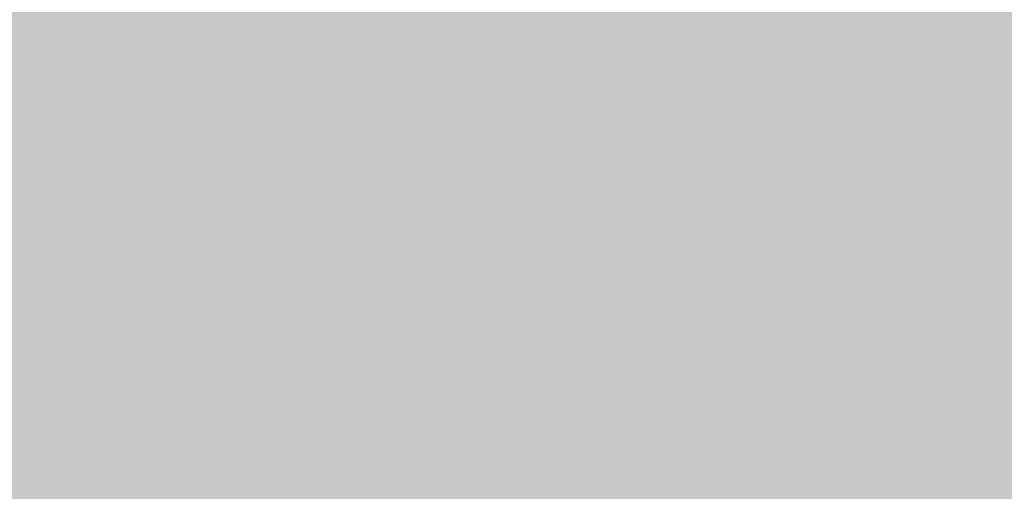
# Model space of a CAD drawing. Units: millimetres. Extents: x 0 to 2267, y 0 to 1823.
# Tile 201 of 256: x 1838.83 to 1841.442, y 1128.399 to 1129.649. Entities that reach past the tile are written whole.
import ezdxf

# ---------------------------------------------------------------- set-up
doc = ezdxf.new("R2010")
doc.units = ezdxf.units.MM
doc.header["$MEASUREMENT"] = 0
doc.layers.add('M-HATC', color=252, linetype='Continuous', lineweight=18)

msp = doc.modelspace()

# ---------------------------------------------------------------- hatches: boundary and pattern name
at = {"layer": 'M-HATC'}
h = msp.add_hatch(color=256, dxfattribs=at)
h.dxf.hatch_style = 1
h.paths.add_polyline_path([(2055.771, 1603.062), (1381.0868, 1603.062), (1381.0868, 1598.062), (2055.771, 1598.062)])
h.paths.add_polyline_path([(2055.771, 1598.062), (1381.0868, 1598.062), (1381.0868, 1593.062), (2055.771, 1593.062)])
h.paths.add_polyline_path([(2051.3074, 1536.7609), (1385.5504, 1536.7609), (1385.5504, 1526.7609), (1387.5504, 1526.7609), (1388.5366, 1525.0528), (1385.3319, 1521.2335), (1385.3319, 1521.2226), (2050.2542, 1522.7491), (2048.3212, 1525.0528), (2049.3074, 1526.7609), (2051.3074, 1526.7609)])
edge = h.paths.add_edge_path()
edge.add_arc((1847.5345, 1379.1492), 135, 222.603061, 222.890851, ccw=False)
edge.add_line((1748.1663, 1287.7656), (1683.0921, 1287.7656))
edge.add_arc((1583.7239, 1379.1492), 135, 317.109149, 317.396939, ccw=False)
edge.add_arc((1678.9686, 1290.6707), 5, 222.8909, 317.1091, ccw=False)
edge.add_arc((1774.2133, 1379.1492), 135, 222.603061, 222.890851, ccw=False)
edge.add_line((1674.8451, 1287.7656), (1609.7709, 1287.7656))
edge.add_arc((1510.4027, 1379.1492), 135, 317.109149, 317.396939, ccw=False)
edge.add_arc((1605.6474, 1290.6707), 5, 222.8909, 317.1091, ccw=False)
edge.add_arc((1700.8921, 1379.1492), 135, 222.603061, 222.890851, ccw=False)
edge.add_line((1601.5239, 1287.7656), (1536.4497, 1287.7656))
edge.add_arc((1437.0815, 1379.1492), 135, 317.109149, 317.396939, ccw=False)
edge.add_arc((1532.3262, 1290.6707), 5, 222.8909, 317.1091, ccw=False)
edge.add_arc((1627.5709, 1379.1492), 135, 222.603061, 222.890851, ccw=False)
edge.add_line((1528.2027, 1287.7656), (1505.9289, 1287.7656))
edge.add_spline(control_points=[(1505.9289, 1287.7656), (1504.2622, 1287.7656), (1504.2622, 1282.7656), (1505.9289, 1282.7656)], knot_values=[0, 0, 0, 0, 5, 5, 5, 5], degree=3, periodic=0)
edge.add_line((1505.9289, 1282.7656), (1930.9289, 1282.7656))
edge.add_spline(control_points=[(1930.9289, 1282.7656), (1932.5956, 1282.7656), (1932.5956, 1287.7656), (1930.9289, 1287.7656)], knot_values=[0, 0, 0, 0, 5, 5, 5, 5], degree=3, periodic=0)
edge.add_line((1930.9289, 1287.7656), (1903.0557, 1287.7656))
edge.add_arc((1803.6875, 1379.1492), 135, 317.109149, 317.396939, ccw=False)
edge.add_arc((1898.9322, 1290.6707), 5, 222.8909, 317.1091, ccw=False)
edge.add_arc((1994.1769, 1379.1492), 135, 222.603061, 222.890851, ccw=False)
edge.add_line((1894.8087, 1287.7656), (1829.7345, 1287.7656))
edge.add_arc((1730.3663, 1379.1492), 135, 317.109149, 317.396939, ccw=False)
edge.add_arc((1825.611, 1290.6707), 5, 222.8909, 317.1091, ccw=False)
edge.add_arc((1920.8557, 1379.1492), 135, 222.603061, 222.890851, ccw=False)
edge.add_line((1821.4875, 1287.7656), (1756.4133, 1287.7656))
edge.add_arc((1657.0451, 1379.1492), 135, 317.109149, 317.396939, ccw=False)
edge.add_arc((1752.2898, 1290.6707), 5, 222.8909, 317.1091, ccw=False)
edge = h.paths.add_edge_path()
edge.add_spline(control_points=[(1843.4289, 1227.2475), (1845.0956, 1227.2475), (1845.0956, 1232.2475), (1843.4289, 1232.2475)], knot_values=[0, 0, 0, 0, 5, 5, 5, 5], degree=3, periodic=0)
edge.add_line((1843.4289, 1232.2475), (1593.4289, 1232.2475))
edge.add_spline(control_points=[(1593.4289, 1232.2475), (1591.7622, 1232.2475), (1591.7622, 1227.2475), (1593.4289, 1227.2475)], knot_values=[0, 0, 0, 0, 5, 5, 5, 5], degree=3, periodic=0)
edge.add_line((1593.4289, 1227.2475), (1843.4289, 1227.2475))
h.paths.add_polyline_path([(1905.9289, 1127.4171), (1530.9289, 1127.4171, 0.414214), (1520.9289, 1117.4171), (1530.9289, 1117.4171), (1915.9289, 1117.4171, 0.414214)])
edge = h.paths.add_edge_path()
edge.add_arc((1397.0858, 1498.4078), 12.7299, 90.78215, 190.87871, ccw=False)
edge.add_line((1396.912, 1511.1365), (1428.0097, 1511.3488))
edge.add_line((1428.0097, 1511.3488), (1433.0097, 1511.3488))
edge.add_line((1433.0097, 1511.3488), (1434.439, 1511.3488))
edge.add_arc((1419.474, 1498.0804), 20, 41.561, 74.08211)
edge.add_line((1424.9592, 1517.3135), (1399.9351, 1517.2561))
edge.add_spline(control_points=[(1399.9307, 1517.2561), (1399.884, 1517.2131), (1399.8328, 1517.1689), (1399.7774, 1517.1236)], knot_values=[11.567499, 11.567499, 11.567499, 11.567499, 11.814249, 11.814249, 11.814249, 11.814249], degree=3, periodic=0)
edge.add_spline(control_points=[(1399.6328, 1517.0099), (1399.5831, 1516.9721), (1399.5307, 1516.9338), (1399.4759, 1516.8947)], knot_values=[11.167718, 11.167718, 11.167718, 11.167718, 11.365188, 11.365188, 11.365188, 11.365188], degree=3, periodic=0)
edge.add_spline(control_points=[(1399.3398, 1516.8001), (1399.1514, 1516.6719), (1398.9384, 1516.5377), (1398.704, 1516.3994)], knot_values=[10.376405, 10.376405, 10.376405, 10.376405, 11.00994, 11.00994, 11.00994, 11.00994], degree=3, periodic=0)
edge.add_spline(control_points=[(1398.6572, 1516.3719), (1398.5789, 1516.326), (1398.4983, 1516.2797), (1398.4155, 1516.2331)], knot_values=[10.125175, 10.125175, 10.125175, 10.125175, 10.334406, 10.334406, 10.334406, 10.334406], degree=3, periodic=0)
edge.add_spline(control_points=[(1398.2642, 1516.1487), (1398.196, 1516.1111), (1398.1263, 1516.0732), (1398.0555, 1516.0351)], knot_values=[9.832246, 9.832246, 9.832246, 9.832246, 9.999658, 9.999658, 9.999658, 9.999658], degree=3, periodic=0)
edge.add_spline(control_points=[(1397.9987, 1516.0048), (1397.7312, 1515.8621), (1397.446, 1515.7171), (1397.1466, 1515.5714)], knot_values=[9.161808, 9.161808, 9.161808, 9.161808, 9.787769, 9.787769, 9.787769, 9.787769], degree=3, periodic=0)
edge.add_spline(control_points=[(1397.1466, 1515.5714), (1396.8418, 1515.423), (1396.5222, 1515.274), (1396.1914, 1515.1262)], knot_values=[8.524455, 8.524455, 8.524455, 8.524455, 9.161808, 9.161808, 9.161808, 9.161808], degree=3, periodic=0)
edge.add_spline(control_points=[(1396.0777, 1515.0756), (1395.9854, 1515.0348), (1395.8922, 1514.994), (1395.7983, 1514.9534)], knot_values=[8.275193, 8.275193, 8.275193, 8.275193, 8.451726, 8.451726, 8.451726, 8.451726], degree=3, periodic=0)
edge.add_spline(control_points=[(1395.6018, 1514.8691), (1395.4997, 1514.8257), (1395.3968, 1514.7824), (1395.2932, 1514.7394)], knot_values=[7.962917, 7.962917, 7.962917, 7.962917, 8.152764, 8.152764, 8.152764, 8.152764], degree=3, periodic=0)
edge.add_spline(control_points=[(1395.2116, 1514.7057), (1394.8278, 1514.5475), (1394.4345, 1514.3929), (1394.0364, 1514.2442)], knot_values=[7.21254, 7.21254, 7.21254, 7.21254, 7.913148, 7.913148, 7.913148, 7.913148], degree=3, periodic=0)
edge.add_spline(control_points=[(1394.0364, 1514.2442), (1393.7076, 1514.1214), (1393.3754, 1514.0027), (1393.0427, 1513.8895)], knot_values=[6.633733, 6.633733, 6.633733, 6.633733, 7.21254, 7.21254, 7.21254, 7.21254], degree=3, periodic=0)
edge.add_spline(control_points=[(1392.8214, 1513.815), (1392.7198, 1513.7812), (1392.6181, 1513.7479), (1392.5166, 1513.7152)], knot_values=[6.328796, 6.328796, 6.328796, 6.328796, 6.505493, 6.505493, 6.505493, 6.505493], degree=3, periodic=0)
edge.add_spline(control_points=[(1392.5166, 1513.7152), (1392.3187, 1513.6515), (1392.1212, 1513.59), (1391.9244, 1513.531)], knot_values=[5.984605, 5.984605, 5.984605, 5.984605, 6.328796, 6.328796, 6.328796, 6.328796], degree=3, periodic=0)
edge.add_spline(control_points=[(1391.7915, 1513.4915), (1391.3122, 1513.3501), (1390.8384, 1513.2239), (1390.3784, 1513.1171)], knot_values=[5.066697, 5.066697, 5.066697, 5.066697, 5.907055, 5.907055, 5.907055, 5.907055], degree=3, periodic=0)
edge.add_spline(control_points=[(1390.3784, 1513.1171), (1390.1797, 1513.071), (1389.9836, 1513.0284), (1389.7907, 1512.9899)], knot_values=[4.70367, 4.70367, 4.70367, 4.70367, 5.066695, 5.066695, 5.066695, 5.066695], degree=3, periodic=0)
edge.add_spline(control_points=[(1389.422, 1512.9204), (1389.2459, 1512.8892), (1389.0729, 1512.8617), (1388.9036, 1512.8381)], knot_values=[4.130571, 4.130571, 4.130571, 4.130571, 4.469816, 4.469816, 4.469816, 4.469816], degree=3, periodic=0)
edge.add_spline(control_points=[(1388.9036, 1512.8381), (1388.591, 1512.7946), (1388.2911, 1512.7644), (1388.0071, 1512.7494)], knot_values=[3.504031, 3.504031, 3.504031, 3.504031, 4.130571, 4.130571, 4.130571, 4.130571], degree=3, periodic=0)
edge.add_spline(control_points=[(1387.9356, 1512.7459), (1387.8538, 1512.7423), (1387.7733, 1512.74), (1387.6944, 1512.739)], knot_values=[3.268866, 3.268866, 3.268866, 3.268866, 3.451164, 3.451164, 3.451164, 3.451164], degree=3, periodic=0)
edge.add_spline(control_points=[(1387.3351, 1512.7443), (1387.2076, 1512.7499), (1387.0847, 1512.7597), (1386.967, 1512.7739)], knot_values=[2.670686, 2.670686, 2.670686, 2.670686, 2.984, 2.984, 2.984, 2.984], degree=3, periodic=0)
edge.add_spline(control_points=[(1386.8327, 1512.7922), (1386.8209, 1512.7941), (1386.8092, 1512.7959), (1386.7975, 1512.7979)], knot_values=[2.516981, 2.516981, 2.516981, 2.516981, 2.549528, 2.549528, 2.549528, 2.549528], degree=3, periodic=0)
edge.add_spline(control_points=[(1386.4526, 1512.8735), (1386.4257, 1512.881), (1386.3993, 1512.889), (1386.3733, 1512.8972)], knot_values=[2.095869, 2.095869, 2.095869, 2.095869, 2.17941, 2.17941, 2.17941, 2.17941], degree=3, periodic=0)
edge.add_spline(control_points=[(1386.0691, 1513.0189), (1386.0634, 1513.0217), (1386.0577, 1513.0246), (1386.052, 1513.0275)], knot_values=[1.72453, 1.72453, 1.72453, 1.72453, 1.745933, 1.745933, 1.745933, 1.745933], degree=3, periodic=0)
edge.add_arc((1399.474, 1498.0804), 20, 131.82432, 180)
edge.add_arc((1630.3336, 1505.5484), 250.9708, 181.705176, 236.427975)
edge.add_arc((1605.3399, 1483.3044), 218.7822, 238.660829, 243.34961)
edge.add_arc((1647.0911, 1510.3592), 262.8986, 183.129836, 237.853442, ccw=False)
h.paths.add_polyline_path([(1406.5369, 1391.9644, 0.149382), (1491.5506, 1296.4418, -0.129517)], flags=17)
edge = h.paths.add_edge_path()
edge.add_arc((2037.3838, 1498.0804), 20, 0, 48.26587)
edge.add_spline(control_points=[(2050.6973, 1513.0052), (2050.6512, 1512.9847), (2050.6034, 1512.9655), (2050.5539, 1512.9477)], knot_values=[1.835652, 1.835652, 1.835652, 1.835652, 2.000781, 2.000781, 2.000781, 2.000781], degree=3, periodic=0)
edge.add_spline(control_points=[(2050.4616, 1512.9166), (2050.479, 1512.9221), (2050.4963, 1512.9277), (2050.5133, 1512.9335)], knot_values=[2.045477, 2.045477, 2.045477, 2.045477, 2.101389, 2.101389, 2.101389, 2.101389], degree=3, periodic=0)
edge.add_spline(control_points=[(2050.129, 1512.8342), (2050.1984, 1512.8473), (2050.2657, 1512.8623), (2050.3308, 1512.8792)], knot_values=[2.237629, 2.237629, 2.237629, 2.237629, 2.435841, 2.435841, 2.435841, 2.435841], degree=3, periodic=0)
edge.add_spline(control_points=[(2050.0946, 1512.8278), (2050.1061, 1512.8299), (2050.1176, 1512.832), (2050.129, 1512.8342)], knot_values=[2.435841, 2.435841, 2.435841, 2.435841, 2.468321, 2.468321, 2.468321, 2.468321], degree=3, periodic=0)
edge.add_spline(control_points=[(2049.7843, 1512.7851), (2049.8552, 1512.7922), (2049.9243, 1512.8008), (2049.9917, 1512.8109)], knot_values=[2.563852, 2.563852, 2.563852, 2.563852, 2.748541, 2.748541, 2.748541, 2.748541], degree=3, periodic=0)
edge.add_spline(control_points=[(2049.4052, 1512.7617), (2049.5364, 1512.7653), (2049.6629, 1512.773), (2049.7843, 1512.7851)], knot_values=[2.748541, 2.748541, 2.748541, 2.748541, 3.064882, 3.064882, 3.064882, 3.064882], degree=3, periodic=0)
edge.add_spline(control_points=[(2049.1698, 1512.7597), (2049.2336, 1512.7591), (2049.2965, 1512.7594), (2049.3584, 1512.7606)], knot_values=[3.102309, 3.102309, 3.102309, 3.102309, 3.2503, 3.2503, 3.2503, 3.2503], degree=3, periodic=0)
edge.add_spline(control_points=[(2048.8573, 1512.7691), (2048.9638, 1512.7638), (2049.068, 1512.7606), (2049.1698, 1512.7597)], knot_values=[3.2503, 3.2503, 3.2503, 3.2503, 3.486069, 3.486069, 3.486069, 3.486069], degree=3, periodic=0)
edge.add_spline(control_points=[(2048.6924, 1512.7789), (2048.3729, 1512.8009), (2048.0345, 1512.8411), (2047.6817, 1512.897)], knot_values=[3.606429, 3.606429, 3.606429, 3.606429, 4.2989, 4.2989, 4.2989, 4.2989], degree=3, periodic=0)
edge.add_spline(control_points=[(2047.6817, 1512.897), (2047.5458, 1512.9185), (2047.4077, 1512.9424), (2047.2678, 1512.9685)], knot_values=[4.2989, 4.2989, 4.2989, 4.2989, 4.565769, 4.565769, 4.565769, 4.565769], degree=3, periodic=0)
edge.add_spline(control_points=[(2047.2678, 1512.9685), (2047.1449, 1512.9914), (2047.0207, 1513.016), (2046.8951, 1513.0422)], knot_values=[4.565769, 4.565769, 4.565769, 4.565769, 4.799971, 4.799971, 4.799971, 4.799971], degree=3, periodic=0)
edge.add_spline(control_points=[(2046.8951, 1513.0422), (2046.5286, 1513.1188), (2046.1513, 1513.209), (2045.7676, 1513.3107)], knot_values=[4.799971, 4.799971, 4.799971, 4.799971, 5.483718, 5.483718, 5.483718, 5.483718], degree=3, periodic=0)
edge.add_spline(control_points=[(2045.7676, 1513.3107), (2045.3724, 1513.4154), (2044.9704, 1513.5322), (2044.5662, 1513.6588)], knot_values=[5.483718, 5.483718, 5.483718, 5.483718, 6.187866, 6.187866, 6.187866, 6.187866], degree=3, periodic=0)
edge.add_spline(control_points=[(2044.5662, 1513.6588), (2044.4149, 1513.7061), (2044.2633, 1513.7549), (2044.1116, 1513.8048)], knot_values=[6.187866, 6.187866, 6.187866, 6.187866, 6.451551, 6.451551, 6.451551, 6.451551], degree=3, periodic=0)
edge.add_spline(control_points=[(2044.1116, 1513.8048), (2043.9967, 1513.8427), (2043.8817, 1513.8813), (2043.7668, 1513.9205)], knot_values=[6.451551, 6.451551, 6.451551, 6.451551, 6.651434, 6.651434, 6.651434, 6.651434], degree=3, periodic=0)
edge.add_spline(control_points=[(2043.7668, 1513.9205), (2043.3716, 1514.0554), (2042.9774, 1514.1979), (2042.5886, 1514.3458)], knot_values=[6.651434, 6.651434, 6.651434, 6.651434, 7.338879, 7.338879, 7.338879, 7.338879], degree=3, periodic=0)
edge.add_spline(control_points=[(2042.5886, 1514.3458), (2042.1643, 1514.5071), (2041.7465, 1514.6749), (2041.3409, 1514.846)], knot_values=[7.338879, 7.338879, 7.338879, 7.338879, 8.089209, 8.089209, 8.089209, 8.089209], degree=3, periodic=0)
edge.add_spline(control_points=[(2041.3409, 1514.846), (2041.1028, 1514.9465), (2040.869, 1515.0481), (2040.6405, 1515.1502)], knot_values=[8.089209, 8.089209, 8.089209, 8.089209, 8.529587, 8.529587, 8.529587, 8.529587], degree=3, periodic=0)
edge.add_spline(control_points=[(2040.51, 1515.2089), (2040.0824, 1515.4022), (2039.6747, 1515.5971), (2039.295, 1515.7894)], knot_values=[8.613818, 8.613818, 8.613818, 8.613818, 9.44571, 9.44571, 9.44571, 9.44571], degree=3, periodic=0)
edge.add_spline(control_points=[(2039.295, 1515.7894), (2039.0618, 1515.9075), (2038.8391, 1516.0246), (2038.6288, 1516.1398)], knot_values=[9.44571, 9.44571, 9.44571, 9.44571, 9.956404, 9.956404, 9.956404, 9.956404], degree=3, periodic=0)
edge.add_spline(control_points=[(2038.6288, 1516.1398), (2038.5187, 1516.2001), (2038.4121, 1516.2598), (2038.309, 1516.3189)], knot_values=[9.956404, 9.956404, 9.956404, 9.956404, 10.223542, 10.223542, 10.223542, 10.223542], degree=3, periodic=0)
edge.add_spline(control_points=[(2038.309, 1516.3189), (2038.2138, 1516.3735), (2038.1216, 1516.4276), (2038.0328, 1516.481)], knot_values=[10.223542, 10.223542, 10.223542, 10.223542, 10.47051, 10.47051, 10.47051, 10.47051], degree=3, periodic=0)
edge.add_spline(control_points=[(2038.0328, 1516.481), (2037.7855, 1516.6296), (2037.5639, 1516.773), (2037.3722, 1516.909)], knot_values=[10.47051, 10.47051, 10.47051, 10.47051, 11.15767, 11.15767, 11.15767, 11.15767], degree=3, periodic=0)
edge.add_spline(control_points=[(2037.3722, 1516.909), (2037.2789, 1516.9752), (2037.1927, 1517.0396), (2037.1142, 1517.102)], knot_values=[11.15767, 11.15767, 11.15767, 11.15767, 11.49227, 11.49227, 11.49227, 11.49227], degree=3, periodic=0)
edge.add_spline(control_points=[(2036.8564, 1517.3259), (2036.9148, 1517.2692), (2036.9814, 1517.2103), (2037.0557, 1517.1492)], knot_values=[11.577341, 11.577341, 11.577341, 11.577341, 11.91035, 11.91035, 11.91035, 11.91035], degree=3, periodic=0)
edge.add_spline(control_points=[(2036.8074, 1517.3748), (2036.823, 1517.3587), (2036.8393, 1517.3424), (2036.8564, 1517.3259)], knot_values=[11.91035, 11.91035, 11.91035, 11.91035, 12.007402, 12.007402, 12.007402, 12.007402], degree=3, periodic=0)
edge.add_spline(control_points=[(2036.7017, 1517.494), (2036.7104, 1517.483), (2036.7196, 1517.4719), (2036.7291, 1517.4606)], knot_values=[12.184155, 12.184155, 12.184155, 12.184155, 12.255409, 12.255409, 12.255409, 12.255409], degree=3, periodic=0)
edge.add_spline(control_points=[(2036.6159, 1517.6205), (2036.62, 1517.613), (2036.6243, 1517.6055), (2036.6289, 1517.5979)], knot_values=[12.487913, 12.487913, 12.487913, 12.487913, 12.541035, 12.541035, 12.541035, 12.541035], degree=3, periodic=0)
edge.add_spline(control_points=[(2036.5635, 1517.786), (2036.5637, 1517.7794), (2036.5642, 1517.7726), (2036.565, 1517.7658)], knot_values=[12.911761, 12.911761, 12.911761, 12.911761, 12.968286, 12.968286, 12.968286, 12.968286], degree=3, periodic=0)
edge.add_spline(control_points=[(2036.6166, 1517.9304), (2036.6125, 1517.9259), (2036.6086, 1517.9212), (2036.6049, 1517.9165)], knot_values=[13.382527, 13.382527, 13.382527, 13.382527, 13.433791, 13.433791, 13.433791, 13.433791], degree=3, periodic=0)
edge.add_spline(control_points=[(2036.749, 1518.017), (2036.7361, 1518.0116), (2036.7239, 1518.006), (2036.7124, 1518.0002)], knot_values=[13.726299, 13.726299, 13.726299, 13.726299, 13.809928, 13.809928, 13.809928, 13.809928], degree=3, periodic=0)
edge.add_spline(control_points=[(2036.8604, 1518.0528), (2036.8386, 1518.0474), (2036.8181, 1518.0416), (2036.7988, 1518.0353)], knot_values=[13.910887, 13.910887, 13.910887, 13.910887, 14.02153, 14.02153, 14.02153, 14.02153], degree=3, periodic=0)
edge.add_line((2036.9639, 1518.0804), (2032.3838, 1518.0804))
edge.add_line((2032.3838, 1518.0804), (2027.3838, 1518.0804))
edge.add_line((2027.3838, 1518.0804), (2022.3838, 1518.0804))
edge.add_line((2022.3838, 1518.0804), (2017.3838, 1518.0804))
edge.add_arc((2017.3838, 1498.0804), 20, 90, 138.439)
edge.add_line((2002.4188, 1511.3488), (2003.8481, 1511.3488))
edge.add_line((2003.8481, 1511.3488), (2008.8481, 1511.3488))
edge.add_line((2008.8481, 1511.3488), (2039.772, 1511.1377))
edge.add_arc((2039.772, 1498.4078), 12.7299, -10.87871, 90, ccw=False)
edge.add_arc((1789.7668, 1510.3592), 262.8986, 302.146558, 356.870164, ccw=False)
edge.add_arc((1831.5179, 1483.3044), 218.7822, 296.65039, 301.339171)
edge.add_arc((1806.5242, 1505.5484), 250.9708, 303.572025, 358.294824)
h.paths.add_polyline_path([(2030.321, 1391.9644, -0.129517), (1945.3072, 1296.4418, 0.149382)], flags=17)
edge = h.paths.add_edge_path()
edge.add_spline(control_points=[(2037.2464, 1518.0821), (2037.2898, 1518.081), (2037.3355, 1518.0804), (2037.3838, 1518.0804)], knot_values=[0.000012, 0.000012, 0.000012, 0.000012, 0.144754, 0.144754, 0.144754, 0.144754], degree=3, periodic=0)
edge.add_line((2037.3357, 1518.0804), (2037.0096, 1518.0804))
edge.add_spline(control_points=[(2037.0096, 1518.0804), (2036.9822, 1518.0768), (2036.956, 1518.0727), (2036.9312, 1518.0681)], knot_values=[14.13465, 14.13465, 14.13465, 14.13465, 14.247197, 14.247197, 14.247197, 14.247197], degree=3, periodic=0)
edge.add_spline(control_points=[(2036.9312, 1518.0681), (2036.9276, 1518.0674), (2036.9241, 1518.0667), (2036.9205, 1518.0661)], knot_values=[14.118315, 14.118315, 14.118315, 14.118315, 14.13465, 14.13465, 14.13465, 14.13465], degree=3, periodic=0)
edge.add_spline(control_points=[(2036.9205, 1518.0661), (2036.9118, 1518.0644), (2036.9032, 1518.0626), (2036.8948, 1518.0608)], knot_values=[14.078086, 14.078086, 14.078086, 14.078086, 14.118315, 14.118315, 14.118315, 14.118315], degree=3, periodic=0)
edge.add_spline(control_points=[(2036.8948, 1518.0608), (2036.883, 1518.0583), (2036.8716, 1518.0556), (2036.8604, 1518.0528)], knot_values=[14.02153, 14.02153, 14.02153, 14.02153, 14.078086, 14.078086, 14.078086, 14.078086], degree=3, periodic=0)
edge.add_spline(control_points=[(2036.8604, 1518.0528), (2036.8386, 1518.0474), (2036.8181, 1518.0416), (2036.7988, 1518.0353)], knot_values=[13.910887, 13.910887, 13.910887, 13.910887, 14.02153, 14.02153, 14.02153, 14.02153], degree=3, periodic=0)
edge.add_spline(control_points=[(2036.7988, 1518.0353), (2036.7981, 1518.035), (2036.7974, 1518.0348), (2036.7967, 1518.0346)], knot_values=[13.906906, 13.906906, 13.906906, 13.906906, 13.910887, 13.910887, 13.910887, 13.910887], degree=3, periodic=0)
edge.add_spline(control_points=[(2036.7967, 1518.0346), (2036.7882, 1518.0318), (2036.7799, 1518.0289), (2036.7719, 1518.0259)], knot_values=[13.857826, 13.857826, 13.857826, 13.857826, 13.906906, 13.906906, 13.906906, 13.906906], degree=3, periodic=0)
edge.add_spline(control_points=[(2036.7719, 1518.0259), (2036.764, 1518.023), (2036.7564, 1518.02), (2036.749, 1518.017)], knot_values=[13.809928, 13.809928, 13.809928, 13.809928, 13.857826, 13.857826, 13.857826, 13.857826], degree=3, periodic=0)
edge.add_spline(control_points=[(2036.749, 1518.017), (2036.7361, 1518.0116), (2036.7239, 1518.006), (2036.7124, 1518.0002)], knot_values=[13.726299, 13.726299, 13.726299, 13.726299, 13.809928, 13.809928, 13.809928, 13.809928], degree=3, periodic=0)
edge.add_spline(control_points=[(2036.7124, 1518.0002), (2036.7121, 1518), (2036.7118, 1517.9999), (2036.7115, 1517.9997)], knot_values=[13.723993, 13.723993, 13.723993, 13.723993, 13.726299, 13.726299, 13.726299, 13.726299], degree=3, periodic=0)
edge.add_spline(control_points=[(2036.7115, 1517.9997), (2036.7063, 1517.9971), (2036.7013, 1517.9944), (2036.6965, 1517.9917)], knot_values=[13.686536, 13.686536, 13.686536, 13.686536, 13.723993, 13.723993, 13.723993, 13.723993], degree=3, periodic=0)
edge.add_spline(control_points=[(2036.6965, 1517.9917), (2036.6919, 1517.9891), (2036.6874, 1517.9865), (2036.6831, 1517.9839)], knot_values=[13.651251, 13.651251, 13.651251, 13.651251, 13.686536, 13.686536, 13.686536, 13.686536], degree=3, periodic=0)
edge.add_spline(control_points=[(2036.6831, 1517.9839), (2036.6764, 1517.9798), (2036.67, 1517.9757), (2036.6639, 1517.9714)], knot_values=[13.596804, 13.596804, 13.596804, 13.596804, 13.651251, 13.651251, 13.651251, 13.651251], degree=3, periodic=0)
edge.add_spline(control_points=[(2036.6639, 1517.9714), (2036.6636, 1517.9712), (2036.6633, 1517.9709), (2036.6629, 1517.9707)], knot_values=[13.593956, 13.593956, 13.593956, 13.593956, 13.596804, 13.596804, 13.596804, 13.596804], degree=3, periodic=0)
edge.add_spline(control_points=[(2036.6629, 1517.9707), (2036.6603, 1517.9689), (2036.6577, 1517.967), (2036.6552, 1517.9651)], knot_values=[13.570322, 13.570322, 13.570322, 13.570322, 13.593956, 13.593956, 13.593956, 13.593956], degree=3, periodic=0)
edge.add_spline(control_points=[(2036.6552, 1517.9651), (2036.6525, 1517.9631), (2036.6499, 1517.9611), (2036.6474, 1517.9591)], knot_values=[13.545477, 13.545477, 13.545477, 13.545477, 13.570322, 13.570322, 13.570322, 13.570322], degree=3, periodic=0)
edge.add_spline(control_points=[(2036.6474, 1517.9591), (2036.6472, 1517.9589), (2036.6471, 1517.9588), (2036.6469, 1517.9587)], knot_values=[13.543931, 13.543931, 13.543931, 13.543931, 13.545477, 13.545477, 13.545477, 13.545477], degree=3, periodic=0)
edge.add_spline(control_points=[(2036.6469, 1517.9587), (2036.6412, 1517.9541), (2036.6358, 1517.9494), (2036.6307, 1517.9447)], knot_values=[13.488237, 13.488237, 13.488237, 13.488237, 13.543931, 13.543931, 13.543931, 13.543931], degree=3, periodic=0)
edge.add_spline(control_points=[(2036.6307, 1517.9447), (2036.6282, 1517.9423), (2036.6257, 1517.9399), (2036.6233, 1517.9374)], knot_values=[13.460307, 13.460307, 13.460307, 13.460307, 13.488237, 13.488237, 13.488237, 13.488237], degree=3, periodic=0)
edge.add_spline(control_points=[(2036.6233, 1517.9374), (2036.6215, 1517.9356), (2036.6198, 1517.9338), (2036.6181, 1517.932)], knot_values=[13.439712, 13.439712, 13.439712, 13.439712, 13.460307, 13.460307, 13.460307, 13.460307], degree=3, periodic=0)
edge.add_spline(control_points=[(2036.6181, 1517.932), (2036.6176, 1517.9315), (2036.6171, 1517.9309), (2036.6166, 1517.9304)], knot_values=[13.433791, 13.433791, 13.433791, 13.433791, 13.439712, 13.439712, 13.439712, 13.439712], degree=3, periodic=0)
edge.add_spline(control_points=[(2036.6166, 1517.9304), (2036.6125, 1517.9259), (2036.6086, 1517.9212), (2036.6049, 1517.9165)], knot_values=[13.382527, 13.382527, 13.382527, 13.382527, 13.433791, 13.433791, 13.433791, 13.433791], degree=3, periodic=0)
edge.add_spline(control_points=[(2036.6049, 1517.9165), (2036.6026, 1517.9135), (2036.6004, 1517.9104), (2036.5982, 1517.9074)], knot_values=[13.350017, 13.350017, 13.350017, 13.350017, 13.382527, 13.382527, 13.382527, 13.382527], degree=3, periodic=0)
edge.add_spline(control_points=[(2036.5982, 1517.9074), (2036.5972, 1517.9059), (2036.5962, 1517.9043), (2036.5952, 1517.9028)], knot_values=[13.333922, 13.333922, 13.333922, 13.333922, 13.350017, 13.350017, 13.350017, 13.350017], degree=3, periodic=0)
edge.add_spline(control_points=[(2036.5952, 1517.9028), (2036.5945, 1517.9018), (2036.5939, 1517.9009), (2036.5933, 1517.8999)], knot_values=[13.323828, 13.323828, 13.323828, 13.323828, 13.333922, 13.333922, 13.333922, 13.333922], degree=3, periodic=0)
edge.add_spline(control_points=[(2036.5933, 1517.8999), (2036.5905, 1517.8955), (2036.5879, 1517.8909), (2036.5855, 1517.8864)], knot_values=[13.277545, 13.277545, 13.277545, 13.277545, 13.323828, 13.323828, 13.323828, 13.323828], degree=3, periodic=0)
edge.add_spline(control_points=[(2036.5855, 1517.8864), (2036.5836, 1517.8827), (2036.5817, 1517.8789), (2036.5801, 1517.8751)], knot_values=[13.240119, 13.240119, 13.240119, 13.240119, 13.277545, 13.277545, 13.277545, 13.277545], degree=3, periodic=0)
edge.add_spline(control_points=[(2036.5801, 1517.8751), (2036.5795, 1517.8739), (2036.579, 1517.8727), (2036.5785, 1517.8715)], knot_values=[13.228211, 13.228211, 13.228211, 13.228211, 13.240119, 13.240119, 13.240119, 13.240119], degree=3, periodic=0)
edge.add_spline(control_points=[(2036.5785, 1517.8715), (2036.578, 1517.8702), (2036.5774, 1517.869), (2036.5769, 1517.8677)], knot_values=[13.215717, 13.215717, 13.215717, 13.215717, 13.228211, 13.228211, 13.228211, 13.228211], degree=3, periodic=0)
edge.add_spline(control_points=[(2036.5769, 1517.8677), (2036.5755, 1517.864), (2036.5741, 1517.8603), (2036.5729, 1517.8565)], knot_values=[13.179847, 13.179847, 13.179847, 13.179847, 13.215717, 13.215717, 13.215717, 13.215717], degree=3, periodic=0)
edge.add_spline(control_points=[(2036.5729, 1517.8565), (2036.5713, 1517.8515), (2036.5699, 1517.8464), (2036.5687, 1517.8413)], knot_values=[13.132017, 13.132017, 13.132017, 13.132017, 13.179847, 13.179847, 13.179847, 13.179847], degree=3, periodic=0)
edge.add_spline(control_points=[(2036.5687, 1517.8413), (2036.5684, 1517.8402), (2036.5682, 1517.8392), (2036.568, 1517.8382)], knot_values=[13.122482, 13.122482, 13.122482, 13.122482, 13.132017, 13.132017, 13.132017, 13.132017], degree=3, periodic=0)
edge.add_spline(control_points=[(2036.568, 1517.8382), (2036.5676, 1517.8363), (2036.5672, 1517.8345), (2036.5669, 1517.8327)], knot_values=[13.105592, 13.105592, 13.105592, 13.105592, 13.122482, 13.122482, 13.122482, 13.122482], degree=3, periodic=0)
edge.add_spline(control_points=[(2036.5669, 1517.8327), (2036.5662, 1517.8292), (2036.5657, 1517.8257), (2036.5652, 1517.8222)], knot_values=[13.074063, 13.074063, 13.074063, 13.074063, 13.105592, 13.105592, 13.105592, 13.105592], degree=3, periodic=0)
edge.add_spline(control_points=[(2036.5652, 1517.8222), (2036.5652, 1517.8222), (2036.5652, 1517.8222), (2036.5652, 1517.8222)], knot_values=[13.074043, 13.074043, 13.074043, 13.074043, 13.074063, 13.074063, 13.074063, 13.074063], degree=3, periodic=0)
edge.add_spline(control_points=[(2036.5652, 1517.8222), (2036.5644, 1517.8164), (2036.5639, 1517.8106), (2036.5636, 1517.8046)], knot_values=[13.021884, 13.021884, 13.021884, 13.021884, 13.074043, 13.074043, 13.074043, 13.074043], degree=3, periodic=0)
edge.add_spline(control_points=[(2036.5636, 1517.8046), (2036.5636, 1517.804), (2036.5636, 1517.8034), (2036.5635, 1517.8028)], knot_values=[13.01674, 13.01674, 13.01674, 13.01674, 13.021884, 13.021884, 13.021884, 13.021884], degree=3, periodic=0)
edge.add_spline(control_points=[(2036.5635, 1517.8028), (2036.5634, 1517.8005), (2036.5634, 1517.7982), (2036.5634, 1517.7958)], knot_values=[12.996438, 12.996438, 12.996438, 12.996438, 13.01674, 13.01674, 13.01674, 13.01674], degree=3, periodic=0)
edge.add_spline(control_points=[(2036.5634, 1517.7958), (2036.5633, 1517.7926), (2036.5634, 1517.7893), (2036.5635, 1517.786)], knot_values=[12.968286, 12.968286, 12.968286, 12.968286, 12.996438, 12.996438, 12.996438, 12.996438], degree=3, periodic=0)
edge.add_spline(control_points=[(2036.5635, 1517.786), (2036.5637, 1517.7794), (2036.5642, 1517.7726), (2036.565, 1517.7658)], knot_values=[12.911761, 12.911761, 12.911761, 12.911761, 12.968286, 12.968286, 12.968286, 12.968286], degree=3, periodic=0)
edge.add_spline(control_points=[(2036.565, 1517.7658), (2036.565, 1517.7657), (2036.565, 1517.7656), (2036.565, 1517.7656)], knot_values=[12.911017, 12.911017, 12.911017, 12.911017, 12.911761, 12.911761, 12.911761, 12.911761], degree=3, periodic=0)
edge.add_spline(control_points=[(2036.565, 1517.7656), (2036.5654, 1517.7625), (2036.5658, 1517.7593), (2036.5663, 1517.7562)], knot_values=[12.88528, 12.88528, 12.88528, 12.88528, 12.911017, 12.911017, 12.911017, 12.911017], degree=3, periodic=0)
edge.add_spline(control_points=[(2036.5663, 1517.7562), (2036.5667, 1517.7534), (2036.5672, 1517.7506), (2036.5677, 1517.7478)], knot_values=[12.862519, 12.862519, 12.862519, 12.862519, 12.88528, 12.88528, 12.88528, 12.88528], degree=3, periodic=0)
edge.add_spline(control_points=[(2036.5677, 1517.7478), (2036.5678, 1517.7474), (2036.5679, 1517.7469), (2036.568, 1517.7465)], knot_values=[12.858885, 12.858885, 12.858885, 12.858885, 12.862519, 12.862519, 12.862519, 12.862519], degree=3, periodic=0)
edge.add_spline(control_points=[(2036.568, 1517.7465), (2036.5692, 1517.7399), (2036.5707, 1517.7332), (2036.5724, 1517.7264)], knot_values=[12.8053, 12.8053, 12.8053, 12.8053, 12.858885, 12.858885, 12.858885, 12.858885], degree=3, periodic=0)
edge.add_spline(control_points=[(2036.5724, 1517.7264), (2036.5734, 1517.7226), (2036.5745, 1517.7187), (2036.5756, 1517.7149)], knot_values=[12.775176, 12.775176, 12.775176, 12.775176, 12.8053, 12.8053, 12.8053, 12.8053], degree=3, periodic=0)
edge.add_spline(control_points=[(2036.5756, 1517.7149), (2036.5763, 1517.7125), (2036.577, 1517.7102), (2036.5778, 1517.7078)], knot_values=[12.756759, 12.756759, 12.756759, 12.756759, 12.775176, 12.775176, 12.775176, 12.775176], degree=3, periodic=0)
edge.add_spline(control_points=[(2036.5778, 1517.7078), (2036.5781, 1517.7067), (2036.5784, 1517.7057), (2036.5787, 1517.7047)], knot_values=[12.748742, 12.748742, 12.748742, 12.748742, 12.756759, 12.756759, 12.756759, 12.756759], degree=3, periodic=0)
edge.add_spline(control_points=[(2036.5787, 1517.7047), (2036.5808, 1517.6983), (2036.5831, 1517.6919), (2036.5856, 1517.6854)], knot_values=[12.69959, 12.69959, 12.69959, 12.69959, 12.748742, 12.748742, 12.748742, 12.748742], degree=3, periodic=0)
edge.add_spline(control_points=[(2036.5856, 1517.6854), (2036.5876, 1517.68), (2036.5898, 1517.6746), (2036.5921, 1517.6692)], knot_values=[12.659038, 12.659038, 12.659038, 12.659038, 12.69959, 12.69959, 12.69959, 12.69959], degree=3, periodic=0)
edge.add_spline(control_points=[(2036.5921, 1517.6692), (2036.594, 1517.6648), (2036.5959, 1517.6605), (2036.5979, 1517.6561)], knot_values=[12.626806, 12.626806, 12.626806, 12.626806, 12.659038, 12.659038, 12.659038, 12.659038], degree=3, periodic=0)
edge.add_spline(control_points=[(2036.5979, 1517.6561), (2036.5984, 1517.6551), (2036.5989, 1517.6541), (2036.5993, 1517.6531)], knot_values=[12.619394, 12.619394, 12.619394, 12.619394, 12.626806, 12.626806, 12.626806, 12.626806], degree=3, periodic=0)
edge.add_spline(control_points=[(2036.5993, 1517.6531), (2036.6043, 1517.6424), (2036.6099, 1517.6315), (2036.6159, 1517.6205)], knot_values=[12.541039, 12.541039, 12.541039, 12.541039, 12.619394, 12.619394, 12.619394, 12.619394], degree=3, periodic=0)
edge.add_spline(control_points=[(2036.6159, 1517.6205), (2036.6159, 1517.6205), (2036.6159, 1517.6205), (2036.6159, 1517.6205)], knot_values=[12.541035, 12.541035, 12.541035, 12.541035, 12.541039, 12.541039, 12.541039, 12.541039], degree=3, periodic=0)
edge.add_spline(control_points=[(2036.6159, 1517.6205), (2036.62, 1517.613), (2036.6243, 1517.6055), (2036.6289, 1517.5979)], knot_values=[12.487913, 12.487913, 12.487913, 12.487913, 12.541035, 12.541035, 12.541035, 12.541035], degree=3, periodic=0)
edge.add_spline(control_points=[(2036.6289, 1517.5979), (2036.6326, 1517.5916), (2036.6365, 1517.5853), (2036.6406, 1517.5789)], knot_values=[12.443982, 12.443982, 12.443982, 12.443982, 12.487913, 12.487913, 12.487913, 12.487913], degree=3, periodic=0)
edge.add_spline(control_points=[(2036.6406, 1517.5789), (2036.6414, 1517.5776), (2036.6423, 1517.5763), (2036.6431, 1517.5749)], knot_values=[12.434996, 12.434996, 12.434996, 12.434996, 12.443982, 12.443982, 12.443982, 12.443982], degree=3, periodic=0)
edge.add_spline(control_points=[(2036.6431, 1517.5749), (2036.6531, 1517.5596), (2036.6639, 1517.5439), (2036.6756, 1517.528)], knot_values=[12.329647, 12.329647, 12.329647, 12.329647, 12.434996, 12.434996, 12.434996, 12.434996], degree=3, periodic=0)
edge.add_spline(control_points=[(2036.6756, 1517.528), (2036.6839, 1517.5168), (2036.6925, 1517.5055), (2036.7017, 1517.494)], knot_values=[12.255409, 12.255409, 12.255409, 12.255409, 12.329647, 12.329647, 12.329647, 12.329647], degree=3, periodic=0)
edge.add_spline(control_points=[(2036.7017, 1517.494), (2036.7104, 1517.483), (2036.7196, 1517.4719), (2036.7291, 1517.4606)], knot_values=[12.184155, 12.184155, 12.184155, 12.184155, 12.255409, 12.255409, 12.255409, 12.255409], degree=3, periodic=0)
edge.add_spline(control_points=[(2036.7291, 1517.4606), (2036.7436, 1517.4435), (2036.759, 1517.4262), (2036.7753, 1517.4085)], knot_values=[12.075961, 12.075961, 12.075961, 12.075961, 12.184155, 12.184155, 12.184155, 12.184155], degree=3, periodic=0)
edge.add_spline(control_points=[(2036.7753, 1517.4085), (2036.7763, 1517.4075), (2036.7773, 1517.4064), (2036.7783, 1517.4054)], knot_values=[12.069502, 12.069502, 12.069502, 12.069502, 12.075961, 12.075961, 12.075961, 12.075961], degree=3, periodic=0)
edge.add_spline(control_points=[(2036.7783, 1517.4054), (2036.7877, 1517.3953), (2036.7974, 1517.385), (2036.8074, 1517.3748)], knot_values=[12.007402, 12.007402, 12.007402, 12.007402, 12.069502, 12.069502, 12.069502, 12.069502], degree=3, periodic=0)
edge.add_spline(control_points=[(2036.8074, 1517.3748), (2036.823, 1517.3587), (2036.8393, 1517.3424), (2036.8564, 1517.3259)], knot_values=[11.91035, 11.91035, 11.91035, 11.91035, 12.007402, 12.007402, 12.007402, 12.007402], degree=3, periodic=0)
edge.add_spline(control_points=[(2036.8564, 1517.3259), (2036.9148, 1517.2692), (2036.9814, 1517.2103), (2037.0557, 1517.1492)], knot_values=[11.577341, 11.577341, 11.577341, 11.577341, 11.91035, 11.91035, 11.91035, 11.91035], degree=3, periodic=0)
edge.add_spline(control_points=[(2037.0557, 1517.1492), (2037.0747, 1517.1336), (2037.0942, 1517.1179), (2037.1142, 1517.102)], knot_values=[11.49227, 11.49227, 11.49227, 11.49227, 11.577341, 11.577341, 11.577341, 11.577341], degree=3, periodic=0)
edge.add_spline(control_points=[(2037.1142, 1517.102), (2037.1927, 1517.0396), (2037.2789, 1516.9752), (2037.3722, 1516.909)], knot_values=[11.15767, 11.15767, 11.15767, 11.15767, 11.49227, 11.49227, 11.49227, 11.49227], degree=3, periodic=0)
edge.add_spline(control_points=[(2037.3722, 1516.909), (2037.5639, 1516.773), (2037.7855, 1516.6296), (2038.0328, 1516.481)], knot_values=[10.47051, 10.47051, 10.47051, 10.47051, 11.15767, 11.15767, 11.15767, 11.15767], degree=3, periodic=0)
edge.add_spline(control_points=[(2038.0328, 1516.481), (2038.1216, 1516.4276), (2038.2138, 1516.3735), (2038.309, 1516.3189)], knot_values=[10.223542, 10.223542, 10.223542, 10.223542, 10.47051, 10.47051, 10.47051, 10.47051], degree=3, periodic=0)
edge.add_spline(control_points=[(2038.309, 1516.3189), (2038.4121, 1516.2598), (2038.5187, 1516.2001), (2038.6288, 1516.1398)], knot_values=[9.956404, 9.956404, 9.956404, 9.956404, 10.223542, 10.223542, 10.223542, 10.223542], degree=3, periodic=0)
edge.add_spline(control_points=[(2038.6288, 1516.1398), (2038.8391, 1516.0246), (2039.0618, 1515.9075), (2039.295, 1515.7894)], knot_values=[9.44571, 9.44571, 9.44571, 9.44571, 9.956404, 9.956404, 9.956404, 9.956404], degree=3, periodic=0)
edge.add_spline(control_points=[(2039.295, 1515.7894), (2039.6747, 1515.5971), (2040.0824, 1515.4022), (2040.51, 1515.2089)], knot_values=[8.613818, 8.613818, 8.613818, 8.613818, 9.44571, 9.44571, 9.44571, 9.44571], degree=3, periodic=0)
edge.add_spline(control_points=[(2040.51, 1515.2089), (2040.5533, 1515.1893), (2040.5968, 1515.1697), (2040.6405, 1515.1502)], knot_values=[8.529587, 8.529587, 8.529587, 8.529587, 8.613818, 8.613818, 8.613818, 8.613818], degree=3, periodic=0)
edge.add_spline(control_points=[(2040.6405, 1515.1502), (2040.869, 1515.0481), (2041.1028, 1514.9465), (2041.3409, 1514.846)], knot_values=[8.089209, 8.089209, 8.089209, 8.089209, 8.529587, 8.529587, 8.529587, 8.529587], degree=3, periodic=0)
edge.add_spline(control_points=[(2041.3409, 1514.846), (2041.7465, 1514.6749), (2042.1643, 1514.5071), (2042.5886, 1514.3458)], knot_values=[7.338879, 7.338879, 7.338879, 7.338879, 8.089209, 8.089209, 8.089209, 8.089209], degree=3, periodic=0)
edge.add_spline(control_points=[(2042.5886, 1514.3458), (2042.9774, 1514.1979), (2043.3716, 1514.0554), (2043.7668, 1513.9205)], knot_values=[6.651434, 6.651434, 6.651434, 6.651434, 7.338879, 7.338879, 7.338879, 7.338879], degree=3, periodic=0)
edge.add_spline(control_points=[(2043.7668, 1513.9205), (2043.8817, 1513.8813), (2043.9967, 1513.8427), (2044.1116, 1513.8048)], knot_values=[6.451551, 6.451551, 6.451551, 6.451551, 6.651434, 6.651434, 6.651434, 6.651434], degree=3, periodic=0)
edge.add_spline(control_points=[(2044.1116, 1513.8048), (2044.2633, 1513.7549), (2044.4149, 1513.7061), (2044.5662, 1513.6588)], knot_values=[6.187866, 6.187866, 6.187866, 6.187866, 6.451551, 6.451551, 6.451551, 6.451551], degree=3, periodic=0)
edge.add_spline(control_points=[(2044.5662, 1513.6588), (2044.9704, 1513.5322), (2045.3724, 1513.4154), (2045.7676, 1513.3107)], knot_values=[5.483718, 5.483718, 5.483718, 5.483718, 6.187866, 6.187866, 6.187866, 6.187866], degree=3, periodic=0)
edge.add_spline(control_points=[(2045.7676, 1513.3107), (2046.1513, 1513.209), (2046.5286, 1513.1188), (2046.8951, 1513.0422)], knot_values=[4.799971, 4.799971, 4.799971, 4.799971, 5.483718, 5.483718, 5.483718, 5.483718], degree=3, periodic=0)
edge.add_spline(control_points=[(2046.8951, 1513.0422), (2047.0207, 1513.016), (2047.1449, 1512.9914), (2047.2678, 1512.9685)], knot_values=[4.565769, 4.565769, 4.565769, 4.565769, 4.799971, 4.799971, 4.799971, 4.799971], degree=3, periodic=0)
edge.add_spline(control_points=[(2047.2678, 1512.9685), (2047.4077, 1512.9424), (2047.5458, 1512.9185), (2047.6817, 1512.897)], knot_values=[4.2989, 4.2989, 4.2989, 4.2989, 4.565769, 4.565769, 4.565769, 4.565769], degree=3, periodic=0)
edge.add_spline(control_points=[(2047.6817, 1512.897), (2048.0345, 1512.8411), (2048.3729, 1512.8009), (2048.6924, 1512.7789)], knot_values=[3.606429, 3.606429, 3.606429, 3.606429, 4.2989, 4.2989, 4.2989, 4.2989], degree=3, periodic=0)
edge.add_spline(control_points=[(2048.6924, 1512.7789), (2048.7479, 1512.7751), (2048.8029, 1512.7718), (2048.8573, 1512.7691)], knot_values=[3.486069, 3.486069, 3.486069, 3.486069, 3.606429, 3.606429, 3.606429, 3.606429], degree=3, periodic=0)
edge.add_spline(control_points=[(2048.8573, 1512.7691), (2048.9638, 1512.7638), (2049.068, 1512.7606), (2049.1698, 1512.7597)], knot_values=[3.2503, 3.2503, 3.2503, 3.2503, 3.486069, 3.486069, 3.486069, 3.486069], degree=3, periodic=0)
edge.add_spline(control_points=[(2049.1698, 1512.7597), (2049.2336, 1512.7591), (2049.2965, 1512.7594), (2049.3584, 1512.7606)], knot_values=[3.102309, 3.102309, 3.102309, 3.102309, 3.2503, 3.2503, 3.2503, 3.2503], degree=3, periodic=0)
edge.add_spline(control_points=[(2049.3584, 1512.7606), (2049.3741, 1512.7609), (2049.3897, 1512.7613), (2049.4052, 1512.7617)], knot_values=[3.064882, 3.064882, 3.064882, 3.064882, 3.102309, 3.102309, 3.102309, 3.102309], degree=3, periodic=0)
edge.add_spline(control_points=[(2049.4052, 1512.7617), (2049.5364, 1512.7653), (2049.6629, 1512.773), (2049.7843, 1512.7851)], knot_values=[2.748541, 2.748541, 2.748541, 2.748541, 3.064882, 3.064882, 3.064882, 3.064882], degree=3, periodic=0)
edge.add_spline(control_points=[(2049.7843, 1512.7851), (2049.8552, 1512.7922), (2049.9243, 1512.8008), (2049.9917, 1512.8109)], knot_values=[2.563852, 2.563852, 2.563852, 2.563852, 2.748541, 2.748541, 2.748541, 2.748541], degree=3, periodic=0)
edge.add_spline(control_points=[(2049.9917, 1512.8109), (2050.0265, 1512.8161), (2050.0608, 1512.8218), (2050.0946, 1512.8278)], knot_values=[2.468321, 2.468321, 2.468321, 2.468321, 2.563852, 2.563852, 2.563852, 2.563852], degree=3, periodic=0)
edge.add_spline(control_points=[(2050.0946, 1512.8278), (2050.1061, 1512.8299), (2050.1176, 1512.832), (2050.129, 1512.8342)], knot_values=[2.435841, 2.435841, 2.435841, 2.435841, 2.468321, 2.468321, 2.468321, 2.468321], degree=3, periodic=0)
edge.add_spline(control_points=[(2050.129, 1512.8342), (2050.1984, 1512.8473), (2050.2657, 1512.8623), (2050.3308, 1512.8792)], knot_values=[2.237629, 2.237629, 2.237629, 2.237629, 2.435841, 2.435841, 2.435841, 2.435841], degree=3, periodic=0)
edge.add_spline(control_points=[(2050.3308, 1512.8792), (2050.3754, 1512.8908), (2050.4191, 1512.9032), (2050.4616, 1512.9166)], knot_values=[2.101389, 2.101389, 2.101389, 2.101389, 2.237629, 2.237629, 2.237629, 2.237629], degree=3, periodic=0)
edge.add_spline(control_points=[(2050.4616, 1512.9166), (2050.479, 1512.9221), (2050.4963, 1512.9277), (2050.5133, 1512.9335)], knot_values=[2.045477, 2.045477, 2.045477, 2.045477, 2.101389, 2.101389, 2.101389, 2.101389], degree=3, periodic=0)
edge.add_spline(control_points=[(2050.5133, 1512.9335), (2050.527, 1512.9382), (2050.5405, 1512.9429), (2050.5539, 1512.9477)], knot_values=[2.000781, 2.000781, 2.000781, 2.000781, 2.045477, 2.045477, 2.045477, 2.045477], degree=3, periodic=0)
edge.add_spline(control_points=[(2050.5539, 1512.9477), (2050.6034, 1512.9655), (2050.6512, 1512.9847), (2050.6973, 1513.0052)], knot_values=[1.835652, 1.835652, 1.835652, 1.835652, 2.000781, 2.000781, 2.000781, 2.000781], degree=3, periodic=0)
edge.add_arc((2037.3838, 1498.0804), 20, 48.26587, 90.12993)
edge = h.paths.add_edge_path(flags=16)
edge.add_spline(control_points=[(1386.1389, 1512.9859), (1388.92, 1511.7395), (1398.0387, 1515.5187), (1399.9307, 1517.2561)], knot_values=[1.831046, 1.831046, 1.831046, 1.831046, 11.814249, 11.814249, 11.814249, 11.814249], degree=3, periodic=0)
edge.add_line((1399.9307, 1517.2561), (1393.7435, 1517.2419))
edge.add_arc((1399.474, 1498.0804), 20, 106.6501, 131.8173)
h = msp.add_hatch(color=256, dxfattribs=at)
h.dxf.hatch_style = 1
h.paths.add_polyline_path([(2042.8886, 1580.1796), (2055.771, 1593.062), (1381.0868, 1593.062), (1393.9692, 1580.1796), (1374.086, 1560.2964), (2062.7718, 1560.2964)])
h.paths.add_polyline_path([(1843.4289, 1201.3297), (1843.4289, 1227.2475), (1593.4289, 1227.2475), (1593.4289, 1201.3297, -0.228274), (1574.5989, 1162.2346), (1530.9289, 1127.4171), (1905.9289, 1127.4171), (1862.2589, 1162.2346, -0.228274)])

doc.saveas('drawing.dxf')
